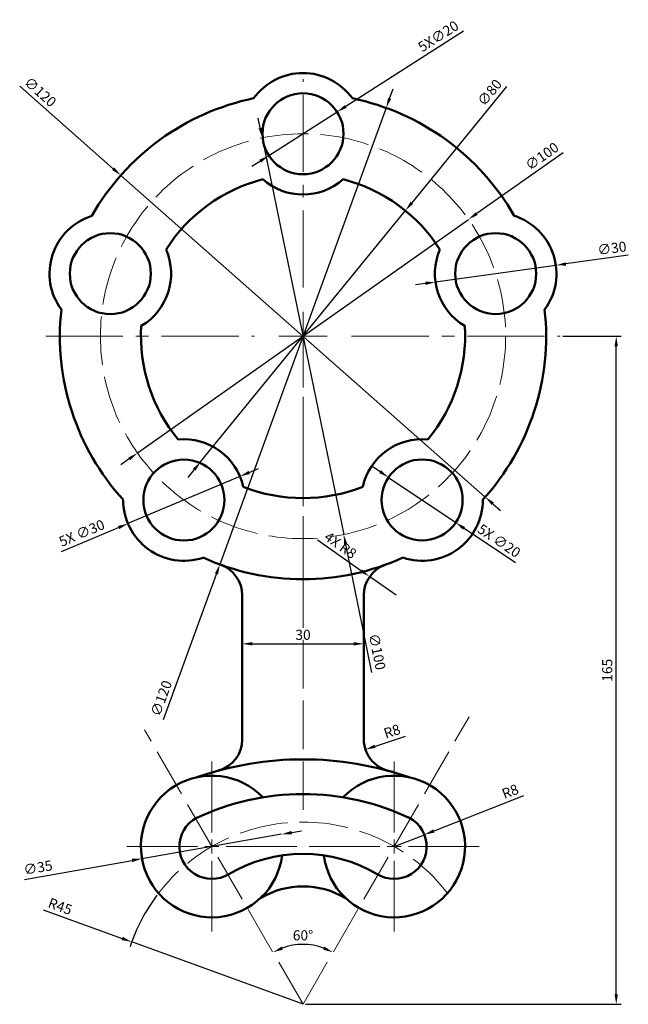
# Model space of a CAD drawing. Units: millimetres. Extents: x 3034 to 3184, y 1574 to 1817.
import ezdxf

# ---------------------------------------------------------------- set-up
doc = ezdxf.new("R2010")
doc.units = ezdxf.units.MM
doc.linetypes.add('ACAD_ISO02W100', pattern=[15, 12, -3])
doc.linetypes.add('CENTER2', pattern=[28.575, 19.05, -3.175, 3.175, -3.175])
for name, color, linetype, lineweight in [('M-CNTR', 4, 'CENTER2', 18), ('M-CONS', 8, 'ACAD_ISO02W100', 18), ('M-DIMS', 2, 'Continuous', 25), ('M-OUTL', 7, 'Continuous', 50)]:
    doc.layers.add(name, color=color, linetype=linetype, lineweight=lineweight)
doc.styles.get("Standard").update_dxf_attribs({"font": 'arial.ttf'})
doc.dimstyles.new('ISO-25', dxfattribs={"dimtxt": 2.5, "dimasz": 2.5, "dimexe": 1.25, "dimexo": 0.625, "dimtad": 1, "dimtxsty": 'Standard', "dimcen": 2.5, "dimadec": 0, "dimazin": 0, "dimtfac": 1, "dimtmove": 0, "dimatfit": 3, "dimfxl": 1, "dimarcsym": 0})

# ---------------------------------------------------------------- blocks, each defined once
blk = doc.blocks.new('*U1')
at = {"layer": 'M-CNTR', "color": 0, "transparency": 16777216}
for p, q in [((0, 12), (0, 63.5)), ((-63.5, 0), (-12, 0)), ((12, 0), (63.5, 0)), ((0, -63.5), (0, -12))]:
    blk.add_line(p, q, dxfattribs=at)
at = {"layer": 'M-CNTR', "color": 0, "linetype": 'Continuous', "transparency": 16777216}
for p, q in [((0, -6), (0, 6)), ((-6, 0), (6, 0))]:
    blk.add_line(p, q, dxfattribs=at)
blk = doc.blocks.new('*U2')
at = {"layer": 'M-CNTR', "color": 0, "transparency": 16777216}
for p, q in [((0, 3.5), (0, 21)), ((-21, 0), (-3.5, 0)), ((3.5, 0), (21, 0)), ((0, -21), (0, -3.5))]:
    blk.add_line(p, q, dxfattribs=at)
at = {"layer": 'M-CNTR', "color": 0, "linetype": 'Continuous', "transparency": 16777216}
for p, q in [((-1.75, 0), (1.75, 0)), ((0, -1.75), (0, 1.75))]:
    blk.add_line(p, q, dxfattribs=at)
blk = doc.blocks.new('*U3')
at = {"layer": 'M-CNTR', "color": 0, "transparency": 16777216}
for p, q in [((0, 3.5), (0, 21)), ((-21, 0), (-3.5, 0)), ((3.5, 0), (21, 0)), ((0, -21), (0, -3.5))]:
    blk.add_line(p, q, dxfattribs=at)
at = {"layer": 'M-CNTR', "color": 0, "linetype": 'Continuous', "transparency": 16777216}
for p, q in [((-1.75, 0), (1.75, 0)), ((0, -1.75), (0, 1.75))]:
    blk.add_line(p, q, dxfattribs=at)
blk = doc.blocks.new('*D4')
at = {"layer": 'Defpoints', "color": 0, "transparency": 16777216}
for p in [(3112.54, 1794.62), (3095.69, 1783.84)]:
    blk.add_point(p, dxfattribs=at)
at = {"layer": 'M-DIMS', "color": 0, "lineweight": -2, "transparency": 16777216}
for p, q in [((3143.71, 1814.56), (3114.65, 1795.97)), ((3095.69, 1783.84), (3112.54, 1794.62)), ((3093.59, 1782.49), (3091.48, 1781.14))]:
    blk.add_line(p, q, dxfattribs=at)
at = {"layer": 'M-DIMS', "color": 0, "transparency": 16777216}
for points in [[(3114.42, 1796.32), (3114.87, 1795.61), (3112.54, 1794.62)], [(3093.36, 1782.84), (3093.81, 1782.14), (3095.69, 1783.84)]]:
    blk.add_solid(points, dxfattribs=at)
at = {"layer": 'M-DIMS', "color": 0, "transparency": 16777216, "insert": (3137.68, 1813.04), "char_height": 2.5, "attachment_point": 5, "rotation": 32.6129}
blk.add_mtext('5X∅20', dxfattribs=at)
blk = doc.blocks.new('*D5')
at = {"layer": 'Defpoints', "color": 0, "transparency": 16777216}
for p in [(3144.96, 1768.07), (3063.28, 1710.39)]:
    blk.add_point(p, dxfattribs=at)
at = {"layer": 'M-DIMS', "color": 0, "lineweight": -2, "transparency": 16777216}
for p, q in [((3168.29, 1784.54), (3147, 1769.51)), ((3063.28, 1710.39), (3144.96, 1768.07)), ((3061.23, 1708.94), (3059.19, 1707.5))]:
    blk.add_line(p, q, dxfattribs=at)
at = {"layer": 'M-DIMS', "color": 0, "transparency": 16777216}
for points in [[(3146.76, 1769.85), (3147.24, 1769.17), (3144.96, 1768.07)], [(3060.99, 1709.28), (3061.47, 1708.6), (3063.28, 1710.39)]]:
    blk.add_solid(points, dxfattribs=at)
at = {"layer": 'M-DIMS', "color": 0, "transparency": 16777216, "insert": (3163.28, 1783.42), "char_height": 2.5, "attachment_point": 5, "rotation": 35.2294}
blk.add_mtext('∅100', dxfattribs=at)
blk = doc.blocks.new('*D6')
at = {"layer": 'Defpoints', "color": 0, "transparency": 16777216}
for p in [(3129.38, 1770.24), (3078.86, 1708.22)]:
    blk.add_point(p, dxfattribs=at)
at = {"layer": 'M-DIMS', "color": 0, "lineweight": -2, "transparency": 16777216}
for p, q in [((3154.33, 1800.87), (3130.96, 1772.18)), ((3078.86, 1708.22), (3129.38, 1770.24)), ((3077.28, 1706.28), (3075.7, 1704.34))]:
    blk.add_line(p, q, dxfattribs=at)
at = {"layer": 'M-DIMS', "color": 0, "transparency": 16777216}
for points in [[(3130.64, 1772.44), (3131.28, 1771.92), (3129.38, 1770.24)], [(3076.95, 1706.54), (3077.6, 1706.01), (3078.86, 1708.22)]]:
    blk.add_solid(points, dxfattribs=at)
at = {"layer": 'M-DIMS', "color": 0, "transparency": 16777216, "insert": (3150.42, 1799.19), "char_height": 2.5, "attachment_point": 5, "rotation": 50.8343}
blk.add_mtext('∅80', dxfattribs=at)
blk = doc.blocks.new('*D7')
at = {"layer": 'Defpoints', "color": 0, "transparency": 16777216}
for p in [(3166.53, 1756.74), (3136.81, 1752.62)]:
    blk.add_point(p, dxfattribs=at)
at = {"layer": 'M-DIMS', "color": 0, "lineweight": -2, "transparency": 16777216}
for p, q in [((3184.4, 1759.21), (3169.01, 1757.08)), ((3136.81, 1752.62), (3166.53, 1756.74)), ((3134.34, 1752.28), (3131.86, 1751.94))]:
    blk.add_line(p, q, dxfattribs=at)
at = {"layer": 'M-DIMS', "color": 0, "transparency": 16777216}
for points in [[(3168.95, 1757.49), (3169.06, 1756.67), (3166.53, 1756.74)], [(3134.28, 1752.69), (3134.39, 1751.87), (3136.81, 1752.62)]]:
    blk.add_solid(points, dxfattribs=at)
at = {"layer": 'M-DIMS', "color": 0, "transparency": 16777216, "insert": (3180.39, 1760.65), "char_height": 2.5, "attachment_point": 5, "rotation": 7.8809}
blk.add_mtext('∅30', dxfattribs=at)
blk = doc.blocks.new('*D8')
at = {"layer": 'Defpoints', "color": 0, "transparency": 16777216}
for p in [(3059.15, 1778.95), (3149.09, 1699.51)]:
    blk.add_point(p, dxfattribs=at)
at = {"layer": 'M-DIMS', "color": 0, "lineweight": -2, "transparency": 16777216}
for p, q in [((3034.2, 1800.98), (3057.27, 1780.6)), ((3149.09, 1699.51), (3059.15, 1778.95)), ((3150.96, 1697.85), (3152.84, 1696.2))]:
    blk.add_line(p, q, dxfattribs=at)
at = {"layer": 'M-DIMS', "color": 0, "transparency": 16777216}
for points in [[(3057.55, 1780.92), (3057, 1780.29), (3059.15, 1778.95)], [(3151.24, 1698.17), (3150.69, 1697.54), (3149.09, 1699.51)]]:
    blk.add_solid(points, dxfattribs=at)
at = {"layer": 'M-DIMS', "color": 0, "transparency": 16777216, "insert": (3039.06, 1799.32), "char_height": 2.5, "attachment_point": 5, "rotation": 318.5474}
blk.add_mtext('∅120', dxfattribs=at)
blk = doc.blocks.new('*D9')
at = {"layer": 'Defpoints', "color": 0, "transparency": 16777216}
for p in [(3098.85, 1616.22), (3064.38, 1610.18)]:
    blk.add_point(p, dxfattribs=at)
at = {"layer": 'M-DIMS', "color": 0, "lineweight": -2, "transparency": 16777216}
for p, q in [((3098.85, 1616.22), (3064.38, 1610.18)), ((3101.32, 1616.65), (3103.78, 1617.09)), ((3035.37, 1605.09), (3061.92, 1609.75))]:
    blk.add_line(p, q, dxfattribs=at)
at = {"layer": 'M-DIMS', "color": 0, "transparency": 16777216}
for points in [[(3101.25, 1617.06), (3101.39, 1616.24), (3098.85, 1616.22)], [(3061.85, 1610.16), (3061.99, 1609.34), (3064.38, 1610.18)]]:
    blk.add_solid(points, dxfattribs=at)
at = {"layer": 'M-DIMS', "color": 0, "transparency": 16777216, "insert": (3038.76, 1607.69), "char_height": 2.5, "attachment_point": 5, "rotation": 9.9452}
blk.add_mtext('∅35', dxfattribs=at)
blk = doc.blocks.new('*D10')
at = {"layer": 'Defpoints', "color": 0, "transparency": 16777216}
for p in [(3127.12, 1639.66), (3119.52, 1637.16)]:
    blk.add_point(p, dxfattribs=at)
at = {"layer": 'M-DIMS', "color": 0, "lineweight": -2, "transparency": 16777216}
blk.add_line((3129.29, 1640.37), (3121.89, 1637.94), dxfattribs=at)
at = {"layer": 'M-DIMS', "color": 0, "transparency": 16777216}
blk.add_solid([(3121.76, 1638.34), (3122.02, 1637.55), (3119.52, 1637.16)], dxfattribs=at)
at = {"layer": 'M-DIMS', "color": 0, "transparency": 16777216, "insert": (3126.19, 1641.36), "char_height": 2.5, "attachment_point": 5, "rotation": 18.1961}
blk.add_mtext('R8', dxfattribs=at)
blk = doc.blocks.new('*D11')
at = {"layer": 'Defpoints', "color": 0, "transparency": 16777216}
for p in [(3134.07, 1616.12), (3126.62, 1613.2)]:
    blk.add_point(p, dxfattribs=at)
at = {"layer": 'M-DIMS', "color": 0, "lineweight": -2, "transparency": 16777216}
for p, q in [((3158.52, 1625.71), (3136.39, 1617.03)), ((3126.62, 1613.2), (3134.07, 1616.12))]:
    blk.add_line(p, q, dxfattribs=at)
at = {"layer": 'M-DIMS', "color": 0, "transparency": 16777216}
blk.add_solid([(3136.24, 1617.42), (3136.55, 1616.64), (3134.07, 1616.12)], dxfattribs=at)
at = {"layer": 'M-DIMS', "color": 0, "transparency": 16777216, "insert": (3155.37, 1626.51), "char_height": 2.5, "attachment_point": 5, "rotation": 21.4072}
blk.add_mtext('R8', dxfattribs=at)
blk = doc.blocks.new('*D12')
at = {"layer": 'Defpoints', "color": 0, "transparency": 16777216}
for p in [(3061.84, 1589.64), (3104.12, 1574.23)]:
    blk.add_point(p, dxfattribs=at)
at = {"layer": 'M-DIMS', "color": 0, "lineweight": -2, "transparency": 16777216}
for p, q in [((3040.03, 1597.58), (3059.49, 1590.49)), ((3104.12, 1574.23), (3061.84, 1589.64))]:
    blk.add_line(p, q, dxfattribs=at)
blk.add_arc((3104.12, 1574.23), 45, 143.2203, 161.5696, dxfattribs=at)
at = {"layer": 'M-DIMS', "color": 0, "transparency": 16777216}
blk.add_solid([(3059.63, 1590.88), (3059.35, 1590.1), (3061.84, 1589.64)], dxfattribs=at)
at = {"layer": 'M-DIMS', "color": 0, "transparency": 16777216, "insert": (3044.08, 1598.12), "char_height": 2.5, "attachment_point": 5, "rotation": 339.978}
blk.add_mtext('R45', dxfattribs=at)
blk = doc.blocks.new('*D13')
at = {"layer": 'Defpoints', "color": 0, "transparency": 16777216}
for p in [(3119.12, 1663.26), (3089.12, 1657.45), (3119.12, 1657.45)]:
    blk.add_point(p, dxfattribs=at)
at = {"layer": 'M-DIMS', "color": 0, "lineweight": -2, "transparency": 16777216}
for p, q in [((3089.12, 1658.07), (3089.12, 1664.51)), ((3119.12, 1658.07), (3119.12, 1664.51)), ((3091.62, 1663.26), (3116.62, 1663.26))]:
    blk.add_line(p, q, dxfattribs=at)
at = {"layer": 'M-DIMS', "color": 0, "transparency": 16777216}
for points in [[(3091.62, 1663.68), (3091.62, 1662.85), (3089.12, 1663.26)], [(3116.62, 1663.68), (3116.62, 1662.85), (3119.12, 1663.26)]]:
    blk.add_solid(points, dxfattribs=at)
at = {"layer": 'M-DIMS', "color": 0, "transparency": 16777216, "insert": (3104.12, 1665.16), "char_height": 2.5, "attachment_point": 5}
blk.add_mtext('30', dxfattribs=at)
blk = doc.blocks.new('*D14')
at = {"layer": 'Defpoints', "color": 0, "transparency": 16777216}
for p in [(3145.09, 1645.2), (3065, 1641.99), (3106.69, 1588.81), (3104.12, 1574.23), (3104.12, 1574.23)]:
    blk.add_point(p, dxfattribs=at)
at = {"layer": 'M-DIMS', "color": 0, "lineweight": -2, "transparency": 16777216}
blk.add_arc((3104.12, 1574.23), 14.81, 69.6847, 110.3153, dxfattribs=at)
at = {"layer": 'M-DIMS', "color": 0, "transparency": 16777216}
for points in [[(3099.15, 1587.74), (3098.8, 1588.49), (3096.71, 1587.05)], [(3109.44, 1588.49), (3109.08, 1587.74), (3111.52, 1587.05)]]:
    blk.add_solid(points, dxfattribs=at)
at = {"layer": 'M-DIMS', "color": 0, "transparency": 16777216, "insert": (3104.12, 1590.94), "char_height": 2.5, "attachment_point": 5}
blk.add_mtext('60°', dxfattribs=at)
blk = doc.blocks.new('FLANGE-BOSS-D30-BORE-D20')
blk.add_circle((12.18, 15), 10)
for start, end in [(35.6853, 144.3147), (228.5904, 311.4096)]:
    blk.add_arc((12.18, 15), 15, start, end)
blk = doc.blocks.new('*D16')
at = {"layer": 'Defpoints', "color": 0, "transparency": 16777216}
for p in [(3167.62, 1739.23), (3181.42, 1739.23), (3104.12, 1574.23)]:
    blk.add_point(p, dxfattribs=at)
at = {"layer": 'M-DIMS', "color": 0, "lineweight": -2, "transparency": 16777216}
for p, q in [((3168.24, 1739.23), (3182.67, 1739.23)), ((3181.42, 1576.73), (3181.42, 1736.73)), ((3104.74, 1574.23), (3182.67, 1574.23))]:
    blk.add_line(p, q, dxfattribs=at)
at = {"layer": 'M-DIMS', "color": 0, "transparency": 16777216}
for points in [[(3181, 1736.73), (3181.83, 1736.73), (3181.42, 1739.23)], [(3181, 1576.73), (3181.83, 1576.73), (3181.42, 1574.23)]]:
    blk.add_solid(points, dxfattribs=at)
at = {"layer": 'M-DIMS', "color": 0, "transparency": 16777216, "insert": (3179.52, 1656.73), "char_height": 2.5, "attachment_point": 5, "rotation": 90}
blk.add_mtext('165', dxfattribs=at)
blk = doc.blocks.new('*D17')
at = {"layer": 'Defpoints', "color": 0, "transparency": 16777216}
for p in [(3124.64, 1795.61), (3083.6, 1682.85)]:
    blk.add_point(p, dxfattribs=at)
at = {"layer": 'M-DIMS', "color": 0, "lineweight": -2, "transparency": 16777216}
for p, q in [((3125.49, 1797.96), (3126.35, 1800.31)), ((3124.64, 1795.61), (3083.6, 1682.85)), ((3069.67, 1644.56), (3082.74, 1680.5))]:
    blk.add_line(p, q, dxfattribs=at)
at = {"layer": 'M-DIMS', "color": 0, "transparency": 16777216}
for points in [[(3125.1, 1798.1), (3125.88, 1797.82), (3124.64, 1795.61)], [(3082.35, 1680.64), (3083.14, 1680.35), (3083.6, 1682.85)]]:
    blk.add_solid(points, dxfattribs=at)
at = {"layer": 'M-DIMS', "color": 0, "transparency": 16777216, "insert": (3069.43, 1649.69), "char_height": 2.5, "attachment_point": 5, "rotation": 70.0022}
blk.add_mtext('∅120', dxfattribs=at)
blk = doc.blocks.new('*D18')
at = {"layer": 'Defpoints', "color": 0, "transparency": 16777216}
for p in [(3094.07, 1788.21), (3114.16, 1690.25)]:
    blk.add_point(p, dxfattribs=at)
at = {"layer": 'M-DIMS', "color": 0, "lineweight": -2, "transparency": 16777216}
for p, q in [((3093.57, 1790.66), (3093.07, 1793.11)), ((3094.07, 1788.21), (3114.16, 1690.25)), ((3121.14, 1656.21), (3114.66, 1687.8))]:
    blk.add_line(p, q, dxfattribs=at)
at = {"layer": 'M-DIMS', "color": 0, "transparency": 16777216}
for points in [[(3093.98, 1790.74), (3093.16, 1790.58), (3094.07, 1788.21)], [(3115.07, 1687.88), (3114.25, 1687.71), (3114.16, 1690.25)]]:
    blk.add_solid(points, dxfattribs=at)
at = {"layer": 'M-DIMS', "color": 0, "transparency": 16777216, "insert": (3122.12, 1661.25), "char_height": 2.5, "attachment_point": 5, "rotation": 281.587}
blk.add_mtext('∅100', dxfattribs=at)
blk = doc.blocks.new('*D19')
at = {"layer": 'Defpoints', "color": 0, "transparency": 16777216}
for p in [(3088.55, 1704.61), (3060.91, 1692.94)]:
    blk.add_point(p, dxfattribs=at)
at = {"layer": 'M-DIMS', "color": 0, "lineweight": -2, "transparency": 16777216}
for p, q in [((3090.85, 1705.58), (3093.15, 1706.56)), ((3088.55, 1704.61), (3060.91, 1692.94)), ((3044.53, 1686.03), (3058.61, 1691.97))]:
    blk.add_line(p, q, dxfattribs=at)
at = {"layer": 'M-DIMS', "color": 0, "transparency": 16777216}
for points in [[(3090.69, 1705.97), (3091.01, 1705.2), (3088.55, 1704.61)], [(3058.44, 1692.36), (3058.77, 1691.59), (3060.91, 1692.94)]]:
    blk.add_solid(points, dxfattribs=at)
at = {"layer": 'M-DIMS', "color": 0, "transparency": 16777216, "insert": (3049.65, 1690.33), "char_height": 2.5, "attachment_point": 5, "rotation": 22.8876}
blk.add_mtext('5X ∅30', dxfattribs=at)
blk = doc.blocks.new('*D20')
at = {"layer": 'Defpoints', "color": 0, "transparency": 16777216}
for p in [(3125.22, 1704.37), (3141.8, 1693.18)]:
    blk.add_point(p, dxfattribs=at)
at = {"layer": 'M-DIMS', "color": 0, "lineweight": -2, "transparency": 16777216}
for p, q in [((3123.15, 1705.77), (3121.07, 1707.17)), ((3125.22, 1704.37), (3141.8, 1693.18)), ((3156.53, 1683.23), (3143.87, 1691.78))]:
    blk.add_line(p, q, dxfattribs=at)
at = {"layer": 'M-DIMS', "color": 0, "transparency": 16777216}
for points in [[(3123.38, 1706.12), (3122.91, 1705.43), (3125.22, 1704.37)], [(3144.1, 1692.13), (3143.63, 1691.44), (3141.8, 1693.18)]]:
    blk.add_solid(points, dxfattribs=at)
at = {"layer": 'M-DIMS', "color": 0, "transparency": 16777216, "insert": (3152.34, 1688.44), "char_height": 2.5, "attachment_point": 5, "rotation": 325.9804}
blk.add_mtext('5X ∅20', dxfattribs=at)
blk = doc.blocks.new('*D21')
at = {"layer": 'Defpoints', "color": 0, "transparency": 16777216}
for p in [(3120.57, 1679.84), (3127.12, 1675.24)]:
    blk.add_point(p, dxfattribs=at)
at = {"layer": 'M-DIMS', "color": 0, "lineweight": -2, "transparency": 16777216}
for p, q in [((3107.68, 1688.9), (3118.53, 1681.28)), ((3127.12, 1675.24), (3120.57, 1679.84))]:
    blk.add_line(p, q, dxfattribs=at)
at = {"layer": 'M-DIMS', "color": 0, "transparency": 16777216}
blk.add_solid([(3118.77, 1681.62), (3118.29, 1680.94), (3120.57, 1679.84)], dxfattribs=at)
at = {"layer": 'M-DIMS', "color": 0, "transparency": 16777216, "insert": (3113.18, 1687.36), "char_height": 2.5, "attachment_point": 5, "rotation": 324.8854}
blk.add_mtext('4X R8', dxfattribs=at)

msp = doc.modelspace()

# ---------------------------------------------------------------- linework, layer by layer
at = {"layer": 'M-CONS'}
for p, q in [((3104.118, 1739.229), (3104.118, 1619.229)), ((3104.118, 1574.229), (3145.09, 1645.195)), ((3104.118, 1574.229), (3064.998, 1641.987))]:
    msp.add_line(p, q, dxfattribs=at)
msp.add_circle((3104.118, 1739.229), 50, dxfattribs=at)
msp.add_arc((3104.118, 1574.229), 45, 37.57546, 142.42454, dxfattribs=at)
at = {"layer": 'M-OUTL'}
for p, q in [((3089.118, 1675.237), (3089.118, 1639.661)), ((3119.118, 1639.661), (3119.118, 1675.237))]:
    msp.add_line(p, q, dxfattribs=at)
for centre, radius, start, end in [((3104.118, 1739.229), 60, 101.71585, 150.28415), ((3104.118, 1739.229), 60, 29.71585, 78.28415), ((3104.118, 1739.229), 40, 104.36151, 147.63849), ((3104.118, 1739.229), 40, 32.36151, 75.63849), ((3104.118, 1739.229), 60, 173.71585, 222.28415), ((3104.118, 1739.229), 60, 317.71585, 6.28415), ((3104.118, 1739.229), 40, 176.36151, 219.63849), ((3104.118, 1739.229), 40, 320.36151, 3.63849), ((3104.118, 1739.229), 40, 248.36151, 291.63849), ((3104.118, 1739.229), 60, 245.71585, 294.28415), ((3081.118, 1675.237), 8, 0, 70.2306), ((3127.118, 1675.237), 8, 109.7694, 180), ((3081.118, 1639.661), 8, 285.17931, 0), ((3127.118, 1639.661), 8, 180, 266.41668), ((3104.118, 1554.885), 79.84, 70.84503, 109.15497), ((3081.618, 1613.2), 17.5, 43.97129, 352.85526), ((3126.618, 1613.2), 17.5, 187.14474, 136.02871), ((3104.118, 1564.894), 61.262, 64.36928, 115.63072), ((3081.618, 1613.2), 8, 109.95079, 301.53765), ((3126.618, 1613.2), 8, 238.46235, 70.04921), ((3104.118, 1575.409), 35.983, 59.06025, 120.93975), ((3104.118, 1582.904), 20.452, 59.04387, 120.95613)]:
    msp.add_arc(centre, radius, start, end, dxfattribs=at)

# ---------------------------------------------------------------- block references
at = {"layer": 'M-CNTR'}
for name, p in [('*U1', (3104.118, 1739.229)), ('*U3', (3081.618, 1613.2)), ('*U2', (3126.618, 1613.2))]:
    msp.add_blockref(name, p, dxfattribs=at)
at = {"layer": 'M-OUTL'}
msp.add_blockref('FLANGE-BOSS-D30-BORE-D20', (3091.934, 1774.229), dxfattribs=at)
for p, rotation in [((3067.065, 1738.457), 71.99999999999544), ((3133.64, 1761.632), 287.9999999999439), ((3093.402, 1703.751), 143.9999999999937), ((3134.547, 1718.074), 215.9999999999915)]:
    msp.add_blockref('FLANGE-BOSS-D30-BORE-D20', p, dxfattribs=dict(at, rotation=rotation))

# ---------------------------------------------------------------- dimensions: what is measured, and where the dimension line sits
at = {"layer": 'M-DIMS'}
dim = msp.add_diameter_dim_2p(p1=(3095.694, 1783.839), p2=(3112.541, 1794.618), text='5X<>', dimstyle='ISO-25', override={"dimclrd": 0, "dimclre": 0, "dimclrt": 0}, dxfattribs=at)
dim.commit()
dim.dimension.update_dxf_attribs({"geometry": '*D4', "text_midpoint": (3138.74, 1811.381), "dimtype": 163})
for p1, p2, override, picture, middle in [((3149.088, 1699.509), (3059.147, 1778.949), {"dimclrd": 0, "dimclre": 0, "dimclrt": 0}, '*D8', (3037.756, 1797.843)), ((3078.855, 1708.216), (3129.38, 1770.242), {"dimclrd": 0, "dimclre": 0, "dimclrt": 0}, '*D6', (3151.951, 1797.949)), ((3124.637, 1795.611), (3083.599, 1682.846), {"dimdec": 0, "dimlfac": 1, "dimrnd": 0, "dimzin": 0, "dimdsep": 46, "dimlunit": 2}, '*D17', (3071.287, 1649.017)), ((3094.075, 1788.21), (3114.16, 1690.248), {"dimdec": 0, "dimlfac": 1, "dimrnd": 0, "dimzin": 0, "dimdsep": 46, "dimlunit": 2}, '*D18', (3120.186, 1660.859)), ((3063.275, 1710.386), (3144.96, 1768.071), {"dimclrd": 0, "dimclre": 0, "dimclrt": 0}, '*D5', (3164.413, 1781.809)), ((3136.812, 1752.623), (3166.529, 1756.736), {"dimclrd": 0, "dimclre": 0, "dimclrt": 0}, '*D7', (3180.661, 1758.692)), ((3098.855, 1616.222), (3064.381, 1610.177), {"dimclrd": 0, "dimclre": 0, "dimclrt": 0}, '*D9', (3039.097, 1605.744))]:
    dim = msp.add_diameter_dim_2p(p1=p1, p2=p2, dimstyle='ISO-25', override=override, dxfattribs=at)
    dim.commit()
    dim.dimension.update_dxf_attribs({"geometry": picture, "text_midpoint": middle, "dimtype": 163})
dim = msp.add_linear_dim(base=(3181.418, 1739.229), p1=(3104.118, 1574.229), p2=(3167.618, 1739.229), angle=90, dimstyle='ISO-25', override={"dimdec": 0, "dimlfac": 1, "dimrnd": 0, "dimzin": 0, "dimdsep": 46, "dimlunit": 2}, dxfattribs=at)
dim.commit()
dim.dimension.update_dxf_attribs({"geometry": '*D16', "text_midpoint": (3179.516, 1656.729)})
for p1, p2, picture, middle in [((3125.219, 1704.373), (3141.795, 1693.183), '*D20', (3151.237, 1686.81)), ((3088.547, 1704.612), (3060.909, 1692.944), '*D19', (3050.416, 1688.514))]:
    dim = msp.add_diameter_dim_2p(p1=p1, p2=p2, text='5X <>', dimstyle='ISO-25', override={"dimdec": 0, "dimlfac": 1, "dimrnd": 0, "dimzin": 0, "dimdsep": 46, "dimlunit": 2}, dxfattribs=at)
    dim.commit()
    dim.dimension.update_dxf_attribs({"geometry": picture, "text_midpoint": middle})
dim = msp.add_radius_dim(center=(3127.118, 1675.237), mpoint=(3120.574, 1679.838), text='4X <>', dimstyle='ISO-25', override={"dimdec": 0, "dimlfac": 1, "dimrnd": 0, "dimzin": 0, "dimdsep": 46, "dimlunit": 2}, dxfattribs=at)
dim.commit()
dim.dimension.update_dxf_attribs({"geometry": '*D21', "text_midpoint": (3113.177, 1687.364)})
dim = msp.add_linear_dim(base=(3119.118, 1663.262), p1=(3089.118, 1657.449), p2=(3119.118, 1657.449), dimstyle='ISO-25', override={"dimclrd": 0, "dimclre": 0, "dimclrt": 0}, dxfattribs=at)
dim.commit()
dim.dimension.update_dxf_attribs({"geometry": '*D13', "text_midpoint": (3104.118, 1665.165)})
dim = msp.add_angular_dim_2l(base=(3106.689, 1588.812), line1=((3104.118, 1574.229), (3145.09, 1645.195)), line2=((3104.118, 1574.229), (3064.998, 1641.987)), dimstyle='ISO-25', override={"dimclrd": 0, "dimclre": 0, "dimclrt": 0}, dxfattribs=at)
dim.commit()
dim.dimension.update_dxf_attribs({"geometry": '*D14', "text_midpoint": (3104.118, 1590.938)})
for center, mpoint, picture, middle in [((3127.118, 1639.661), (3119.518, 1637.162), '*D10', (3126.779, 1639.549)), ((3126.618, 1613.2), (3134.066, 1616.12), '*D11', (3156.063, 1624.744)), ((3104.118, 1574.229), (3061.837, 1589.636), '*D12', (3043.433, 1596.342))]:
    dim = msp.add_radius_dim(center=center, mpoint=mpoint, dimstyle='ISO-25', override={"dimclrd": 0, "dimclre": 0, "dimclrt": 0}, dxfattribs=at)
    dim.commit()
    dim.dimension.update_dxf_attribs({"geometry": picture, "text_midpoint": middle, "dimtype": 164})

doc.saveas('drawing.dxf')
